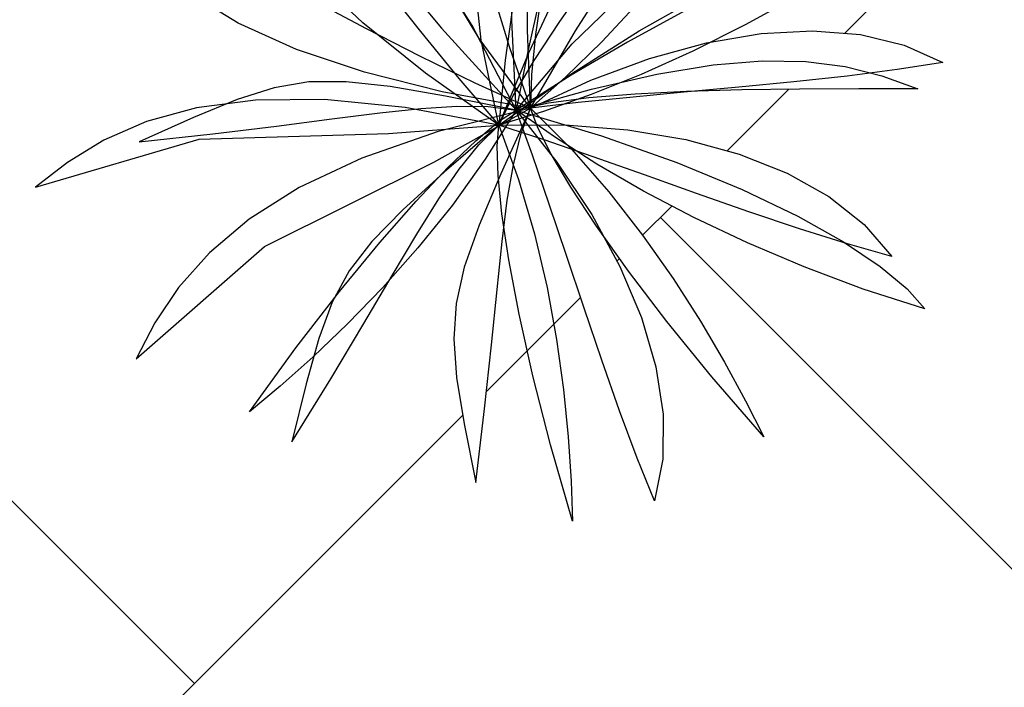
# Model space of a CAD drawing. Units: inches. Extents: x 3590 to 5167, y 65 to 1917.
# Tile 65 of 100: x 4937 to 4968, y 1681 to 1702. Entities that reach past the tile are written whole.
import ezdxf

# ---------------------------------------------------------------- set-up
doc = ezdxf.new("R2010")
doc.units = ezdxf.units.IN
doc.layers.add('A-FLOR-PATT', color=8, linetype='Continuous', lineweight=13)
doc.layers.add('L-PLNT', color=94, linetype='Continuous', lineweight=18)
doc.layers.add('DIENHOA', color=3, linetype='Continuous')

# ---------------------------------------------------------------- blocks, each defined once
blk = doc.blocks.new('Cay03_mb')
at = {"layer": 'DIENHOA'}
for p, q in [((-240.2, 277.8), (-88.4, 94.9)), ((0.2, 104.9), (1.6, 205.7)), ((-49.6, 98.5), (-104.2, 184.4)), ((37.3, 142.1), (20.5, 67.6)), ((75.9, 75.2), (147, 144.1)), ((217.4, 116.6), (145.5, 77.3)), ((5.4, -7.8), (0.2, 104.9)), ((-88.4, 94.9), (5.4, -7.8)), ((5.4, -7.8), (-49.6, 98.5)), ((5.4, -7.8), (75.9, 75.2)), ((145.5, 77.3), (74.7, 36.1)), ((20.5, 67.6), (5.4, -7.8)), ((253, 48.9), (314.6, 54.1)), ((314.6, 54.1), (369.2, 53.3)), ((369.2, 53.3), (418.6, 46.8)), ((100.3, 18.4), (182.2, 37.2)), ((182.2, 37.2), (253, 48.9)), ((418.6, 46.8), (464.9, 35.2)), ((-254.7, 27.4), (-298.6, 20.1)), ((-208, 27.8), (-254.7, 27.4)), ((-152.7, 21.7), (-208, 27.8)), ((74.7, 36.1), (5.4, -7.8)), ((464.9, 35.2), (510, 19)), ((-298.6, 20.1), (-345, 5.4)), ((-83.4, 9.7), (-152.7, 21.7)), ((5.4, -7.8), (100.3, 18.4)), ((219.6, 15.4), (155, 12.2)), ((289, 17.4), (219.6, 15.4)), ((361.6, 18.5), (289, 17.4)), ((435.8, 18.9), (361.6, 18.5)), ((510, 19), (435.8, 18.9)), ((-345, 5.4), (-399.6, -17.1)), ((5.4, -7.8), (-83.4, 9.7)), ((46.3, 0.9), (5.4, -7.8)), ((96.7, 7.5), (46.3, 0.9)), ((155, 12.2), (96.7, 7.5)), ((-225.8, -18.9), (-165.8, -11.3)), ((-165.8, -11.3), (-114, -5.7)), ((-114, -5.7), (-69, -2.9)), ((-69, -2.9), (-29.6, -3.4)), ((5.4, -7.8), (-33.2, -69.5)), ((-29.6, -3.4), (5.4, -7.8)), ((-16.5, -22.4), (5.4, -7.8)), ((5.4, -7.8), (56.8, -73.3)), ((25.9, -64.4), (5.4, -7.8)), ((5.4, -7.8), (112.8, -40.3)), ((53.5, -41.6), (5.4, -7.8)), ((-399.6, -17.1), (-468, -47.9)), ((-295.3, -27.9), (-225.8, -18.9)), ((-45.1, -46.3), (-16.5, -22.4)), ((-375.6, -37.8), (-295.3, -27.9)), ((-468, -47.9), (-375.6, -37.8)), ((-79.8, -79.6), (-45.1, -46.3)), ((107, -75.7), (53.5, -41.6)), ((112.8, -40.3), (207.5, -73.8)), ((-33.2, -69.5), (-74.6, -127.3)), ((47, -125.9), (25.9, -64.4)), ((56.8, -73.3), (100.4, -139.1)), ((207.5, -73.8), (289.5, -107.6)), ((-120.2, -122.1), (-79.8, -79.6)), ((165.5, -109.6), (107, -75.7)), ((228.7, -142.8), (165.5, -109.6)), ((289.5, -107.6), (359.3, -141.1)), ((-165.9, -174.1), (-120.2, -122.1)), ((-74.6, -127.3), (-117.8, -181.1)), ((68.7, -190.6), (47, -125.9)), ((100.4, -139.1), (135.9, -204.3)), ((296, -174.7), (228.7, -142.8)), ((359.3, -141.1), (416.9, -173.5)), ((-216.3, -235.6), (-165.9, -174.1)), ((-117.8, -181.1), (-162.1, -230.9)), ((367.1, -204.8), (296, -174.7)), ((416.9, -173.5), (462.6, -204.2)), ((90.8, -256.6), (68.7, -190.6)), ((135.9, -204.3), (162.8, -268.3)), ((441.6, -232.7), (367.1, -204.8)), ((462.6, -204.2), (496.5, -232.5)), ((-162.1, -230.9), (-206.3, -276.5)), ((518.9, -257.7), (441.6, -232.7)), ((496.5, -232.5), (518.9, -257.7)), ((-271, -306.6), (-216.3, -235.6)), ((113.1, -322.2), (90.8, -256.6)), ((162.8, -268.3), (181, -330.4)), ((-206.3, -276.5), (-249.6, -317.8)), ((-329.5, -387.1), (-271, -306.6)), ((-249.6, -317.8), (-291, -354.7)), ((135.4, -385.6), (113.1, -322.2)), ((181, -330.4), (190, -390)), ((-291, -354.7), (-329.5, -387.1)), ((157.6, -445), (135.4, -385.6)), ((190, -390), (189.6, -446.3)), ((179.5, -498.7), (157.6, -445)), ((189.6, -446.3), (179.5, -498.7))]:
    blk.add_line(p, q, dxfattribs=at)
for points in [[(23.7, -5.4), (-41, 82.2), (-91.8, 167.1), (-129.7, 249.5), (-155.6, 329.6), (-170.2, 407.8), (-174.7, 484.2), (-169.8, 559.3), (-156.5, 633.1)], [(-156.5, 633.1), (-132.5, 551.3), (-110.5, 470), (-89.8, 389.2), (-69.6, 309), (-49, 229.4), (-27.1, 150.4), (-3.2, 72.1), (23.7, -5.4)], [(-16.4, -26.7), (-38.3, 80), (-48.9, 178.3), (-48.7, 269), (-38.5, 352.6), (-19.1, 429.7), (9, 501), (44.9, 567.1), (87.9, 628.5)], [(87.9, 628.5), (75.5, 544.2), (61.3, 461.2), (46.1, 379.1), (30.8, 297.8), (16.1, 216.9), (2.9, 136), (-8.3, 54.9), (-16.4, -26.7)], [(23.7, -5.4), (19.8, 93), (20.3, 177), (25, 248.5), (34, 309.8), (47.3, 362.7), (64.9, 409.3), (86.8, 451.7), (112.9, 491.9)], [(112.9, 491.9), (96, 419.7), (79.5, 347.4), (63.9, 276.5), (50, 208.4), (38.4, 144.8), (29.7, 86.9), (24.6, 36.3), (23.7, -5.4)], [(-395.6, 473.7), (-347.5, 405.6), (-300.6, 339.5), (-254.3, 275.1), (-208.3, 212.3), (-161.9, 150.9), (-114.8, 90.7), (-66.5, 31.6), (-16.4, -26.7)], [(-16.4, -26.7), (-108.3, 38.6), (-186.9, 101.7), (-252.4, 163.5), (-305.1, 224.4), (-345.4, 285.2), (-373.7, 346.6), (-390.4, 409.2), (-395.6, 473.7)], [(384.3, 437.5), (342.2, 367.8), (298.1, 301.7), (252.6, 239.4), (206.1, 181.1), (159.4, 127.2), (113, 78), (67.6, 33.6), (23.7, -5.4)], [(23.7, -5.4), (79.9, 91.7), (134.1, 176.2), (185.8, 248.4), (234.3, 308.7), (279, 357.3), (319.3, 394.8), (354.6, 421.4), (384.3, 437.5)], [(273.2, 387.3), (227.6, 328.8), (182.3, 270.1), (138.4, 212.3), (97.2, 156.4), (60, 103.4), (27.8, 54.6), (1.9, 10.8), (-16.4, -26.7)], [(-16.4, -26.7), (21.4, 64.2), (57, 140.3), (91.4, 203.3), (125.2, 255.1), (159.5, 297.5), (195, 332.5), (232.7, 361.8), (273.2, 387.3)], [(-530.5, 289.7), (-458.3, 248.1), (-387.9, 207.8), (-318.9, 168.7), (-250.8, 131.1), (-182.9, 94.8), (-114.9, 59.9), (-46.2, 26.5), (23.7, -5.4)], [(23.7, -5.4), (-87.2, 15.2), (-185, 39.6), (-270.3, 68.2), (-343.7, 101.4), (-405.9, 139.7), (-457.3, 183.5), (-498.7, 233.4), (-530.5, 289.7)], [(496.7, 224), (429.4, 178.4), (361.6, 136.9), (294.1, 99.5), (227.5, 66.1), (162.4, 36.7), (99.7, 11.5), (39.8, -9.7), (-16.4, -26.7)], [(-16.4, -26.7), (75.4, 37.9), (160.1, 91.8), (237.3, 135.7), (306.6, 170), (367.6, 195.4), (419.9, 212.5), (463.1, 221.9), (496.7, 224)], [(23.7, -5.4), (99.3, 29.7), (173.2, 57.1), (244.8, 76.7), (313.3, 88.3), (377.9, 91.8), (437.9, 87), (492.7, 73.8), (541.4, 52)], [(541.4, 52), (484.1, 42.9), (421.2, 34.8), (354.4, 27.6), (285.4, 20.9), (216.1, 14.5), (148.2, 8.1), (83.5, 1.6), (23.7, -5.4)], [(-16.4, -26.7), (-134, -4.7), (-235.3, 5.3), (-322, 4.7), (-395.9, -5), (-458.7, -22.3), (-512.3, -45.7), (-558.2, -73.6), (-598.4, -104.7)], [(-471.9, -320.3), (-310.5, -179.3), (-97.7, -73.3), (23.7, -5.4)], [(23.7, -5.4), (-92.3, -34.8), (-188.4, -68.2), (-266.9, -105.1), (-329.9, -144.9), (-379.7, -187), (-418.5, -230.7), (-448.5, -275.3), (-471.9, -320.3)], [(23.7, -5.4), (-13.6, -87.9), (-41.1, -152.6), (-59.6, -205), (-69.9, -250.7), (-72.8, -295), (-69.2, -343.6), (-59.7, -401.9), (-45.3, -475.5)], [(-45.3, -475.5), (-34.1, -383.2), (-25.4, -302.8), (-18.3, -233.1), (-12, -172.9), (-5.6, -121.2), (2, -76.8), (11.4, -38.5), (23.7, -5.4)], [(316.5, -418.1), (251.4, -342.8), (194.8, -273.3), (146.5, -210.2), (106.3, -153.8), (74.1, -104.7), (49.7, -63.4), (32.9, -30.1), (23.7, -5.4)], [(23.7, -5.4), (74.9, -57.1), (121.8, -110.6), (164.3, -165), (202.7, -219.4), (237, -272.9), (267.3, -324.5), (293.7, -373.2), (316.5, -418.1)], [(-598.4, -104.7), (-392.7, -44.4), (-155, -37.4), (-16.4, -26.7)], [(-276.2, -424.4), (-227.3, -345.4), (-185.7, -276.1), (-150, -215.7), (-119.1, -163.8), (-91.5, -119.5), (-66, -82.3), (-41.4, -51.6), (-16.4, -26.7)], [(-16.4, -26.7), (-84.9, -86), (-137, -133.1), (-175.8, -173), (-204.3, -210), (-225.5, -249.1), (-242.5, -294.7), (-258.4, -351.6), (-276.2, -424.4)], [(76.2, -524.2), (48.8, -428.5), (26.6, -341.7), (9.2, -264.1), (-3.6, -196.1), (-12.3, -138), (-17.1, -90.2), (-18.3, -53), (-16.4, -26.7)], [(-16.4, -26.7), (66.9, -26.6), (145.6, -32.7), (218.8, -44.9), (285.8, -63.1), (345.9, -87.1), (398.4, -116.6), (442.6, -151.6), (477.6, -191.8)], [(477.6, -191.8), (421.8, -176), (361.3, -156.9), (297.6, -135.5), (232.2, -112.6), (166.6, -89.4), (102.3, -66.6), (40.8, -45.4), (-16.4, -26.7)], [(-16.4, -26.7), (8.5, -95.1), (28.5, -163.3), (44.3, -230.6), (56.3, -296.1), (65, -359), (70.9, -418.5), (74.5, -473.9), (76.2, -524.2)]]:
    blk.add_lwpolyline(points, dxfattribs=at)

msp = doc.modelspace()

# ---------------------------------------------------------------- hatches: boundary and pattern name
at = {"layer": 'A-FLOR-PATT', "transparency": 33554687}
h = msp.add_hatch(dxfattribs=at)
h.set_pattern_fill('AR-HBONE', color=256, scale=0.2)
h.set_pattern_definition([(45, (-588.972, 0), (0, 28.73682), [60.96, -20.32]), (135, (-574.604, 14.368), (3e-15, 28.73682), [60.96, -20.32])])
h.paths.add_polyline_path([(5071.274, 1796.999), (4933.274, 1796.999), (4933.274, 1753.999), (4962.774, 1753.999, -0.414214), (4928.774, 1719.999), (4933.274, 1718.999), (4933.274, 1334.999), (5071.274, 1334.999)])
h.paths.add_polyline_path([(4951.78, 1521.077), (4951.715, 1521.04), (4951.563, 1520.895)], flags=16)
h.paths.add_polyline_path([(4952.267, 1521.376), (4952.198, 1521.371), (4952.198, 1521.356)], flags=0)
h.paths.add_polyline_path([(4967.051, 1529.728), (4965.231, 1528.694), (4963.411, 1527.714), (4961.756, 1526.851), (4963.589, 1527.449), (4964.036, 1527.478), (4962.975, 1527.249), (4961.76, 1526.852), (4959.792, 1525.834), (4958.005, 1524.895), (4956.24, 1523.93), (4954.504, 1522.919), (4954.129, 1522.682), (4953.361, 1521.997), (4953.366, 1521.998), (4953.605, 1522.064), (4955.106, 1522.761), (4956.921, 1523.434), (4958.678, 1523.915), (4960.358, 1524.2), (4961.945, 1524.286), (4964.171, 1524.108), (4965.958, 1523.309), (4963.863, 1522.976), (4965.187, 1522.499), (4963.366, 1522.497), (4961.545, 1522.487), (4959.764, 1522.461), (4958.304, 1522.419), (4957.974, 1522.388), (4956.307, 1522.232), (4954.718, 1522.071), (4953.251, 1521.899), (4953.525, 1521.623), (4954.331, 1521.379), (4956.243, 1521.23), (4958.039, 1520.93), (4959.684, 1520.483), (4961.16, 1519.896), (4963.107, 1518.8), (4964.393, 1517.325), (4962.973, 1517.726), (4964.558, 1516.661), (4965.407, 1515.708), (4963.507, 1516.322), (4961.68, 1517.005), (4959.935, 1517.745), (4958.282, 1518.528), (4956.732, 1519.343), (4955.295, 1520.175), (4954.672, 1520.572), (4954.513, 1520.627), (4955.658, 1519.318), (4956.703, 1517.982), (4957.644, 1516.647), (4958.485, 1515.334), (4959.55, 1513.524), (4960.438, 1511.769), (4958.841, 1513.62), (4957.452, 1515.325), (4955.819, 1517.459), (4956.665, 1515.448), (4957.111, 1513.923), (4957.447, 1511.714), (4957.076, 1509.793), (4956.538, 1511.11), (4955.992, 1512.569), (4955.444, 1514.125), (4954.898, 1515.735), (4954.357, 1517.356), (4953.824, 1518.943), (4953.305, 1520.452), (4953.065, 1521.116), (4952.971, 1521.146), (4952.949, 1521.086), (4952.73, 1520.199), (4953.37, 1518.024), (4953.757, 1516.373), (4954.051, 1514.765), (4954.264, 1513.221), (4954.471, 1511.131), (4954.497, 1510.402), (4954.409, 1511.76), (4954.264, 1513.221), (4954.051, 1514.765), (4953.757, 1516.373), (4953.37, 1518.024), (4952.877, 1519.698), (4952.716, 1520.141), (4952.533, 1519.059), (4952.374, 1517.789), (4952.219, 1516.312), (4952.046, 1514.6), (4951.833, 1512.626), (4951.557, 1510.363), (4951.203, 1512.168), (4950.852, 1514.339), (4950.985, 1516.376), (4951.66, 1518.286), (4952.593, 1520.481), (4952.357, 1521.13), (4951.855, 1520.328), (4950.839, 1518.908), (4949.777, 1517.587), (4948.916, 1516.617), (4948.111, 1515.256), (4947.089, 1513.554), (4945.889, 1511.615), (4946.326, 1513.402), (4946.562, 1514.249), (4945.528, 1513.327), (4944.581, 1512.531), (4946.018, 1514.508), (4947.204, 1516.048), (4947.893, 1517.313), (4949.307, 1518.764), (4950.414, 1519.767), (4950.451, 1519.806), (4952.267, 1521.376), (4951.645, 1521.493), (4950.404, 1521.18), (4948.044, 1520.359), (4946.119, 1519.452), (4944.572, 1518.475), (4943.35, 1517.443), (4941.997, 1515.92), (4941.661, 1515.275), (4942.813, 1516.99), (4944.572, 1518.475), (4946.119, 1519.452), (4948.044, 1520.359), (4950.404, 1521.18), (4951.645, 1521.493), (4949.647, 1521.868), (4948.6, 1521.756), (4947.126, 1521.57), (4945.42, 1521.348), (4943.45, 1521.105), (4941.183, 1520.856), (4942.86, 1521.613), (4943.873, 1522.03), (4942.952, 1521.909), (4941.41, 1521.485), (4939.543, 1520.67), (4938.968, 1520.226), (4940.733, 1521.299), (4942.952, 1521.909), (4943.702, 1522.008), (4945.894, 1522.7), (4947.565, 1522.714), (4948.921, 1522.566), (4951.131, 1522.183), (4950.971, 1522.297), (4948.129, 1523.006), (4946.035, 1523.707), (4944.232, 1524.521), (4942.707, 1525.461), (4941.444, 1526.537), (4940.43, 1527.761), (4939.649, 1529.143), (4941.421, 1528.122), (4943.147, 1527.132), (4944.841, 1526.175), (4946.514, 1525.25), (4948.179, 1524.359), (4948.365, 1524.263), (4946.475, 1526.045), (4945.181, 1527.54), (4944.19, 1529.033), (4943.496, 1530.54), (4943.278, 1531.36), (4942.498, 1531.919), (4943.114, 1531.762), (4942.959, 1533.659), (4944.14, 1531.989), (4944.612, 1531.323), (4946.202, 1530.463), (4947.486, 1529.509), (4948.79, 1528.226), (4950.368, 1526.237), (4949.485, 1528.155), (4948.851, 1530.123), (4948.491, 1532.041), (4948.381, 1533.918), (4948.501, 1535.76), (4948.827, 1537.573), (4949.418, 1535.565), (4949.957, 1533.569), (4950.464, 1531.586), (4950.961, 1529.617), (4951.391, 1527.954), (4951.724, 1530.687), (4952.201, 1532.58), (4952.889, 1534.33), (4953.77, 1535.951), (4954.827, 1537.46), (4954.521, 1535.39), (4954.273, 1533.937), (4955.58, 1535.663), (4956.748, 1536.739), (4956.159, 1534.78), (4955.589, 1532.873), (4955.043, 1531.006), (4954.525, 1529.166), (4954.038, 1527.341), (4953.638, 1525.733), (4953.611, 1525.586), (4953.398, 1524.166), (4953.382, 1524.009), (4954.07, 1525.476), (4954.912, 1527.022), (4956.136, 1528.894), (4957.847, 1530.577), (4959.376, 1531.54), (4958.256, 1530.104), (4957.143, 1528.663), (4956.066, 1527.243), (4955.056, 1525.871), (4954.141, 1524.571), (4953.352, 1523.372), (4953.311, 1523.303), (4953.273, 1522.925), (4953.261, 1522.382), (4954.103, 1523.373), (4954.63, 1524.284), (4955.961, 1526.358), (4957.23, 1528.13), (4958.421, 1529.609), (4960.037, 1531.368), (4961.374, 1532.375), (4962.101, 1532.77), (4961.07, 1531.061), (4959.987, 1529.438), (4958.869, 1527.908), (4958.15, 1527.007), (4959.803, 1528.003), (4961.589, 1528.793), (4963.391, 1529.328), (4965.211, 1529.632)], flags=16)
h.paths.add_polyline_path([(4962.944, 1523.182), (4961.107, 1523.422), (4960.392, 1523.362), (4962.35, 1523.331)], flags=0)
h.paths.add_polyline_path([(5049.541, 1584.551), (5049.476, 1584.515), (5049.325, 1584.37)], flags=16)
h.paths.add_polyline_path([(5050.028, 1584.851), (5049.959, 1584.845), (5049.959, 1584.83)], flags=0)
h.paths.add_polyline_path([(5042.333, 1581.949), (5043.88, 1582.926), (5045.806, 1583.833), (5048.165, 1584.654), (5049.406, 1584.967), (5047.408, 1585.342), (5046.361, 1585.231), (5044.888, 1585.044), (5043.181, 1584.822), (5041.211, 1584.579), (5038.944, 1584.33), (5040.622, 1585.087), (5041.634, 1585.504), (5040.713, 1585.383), (5039.171, 1584.959), (5037.304, 1584.144), (5036.729, 1583.7), (5038.494, 1584.773), (5040.713, 1585.383), (5041.463, 1585.482), (5043.655, 1586.174), (5045.326, 1586.188), (5046.682, 1586.04), (5048.893, 1585.657), (5048.732, 1585.771), (5045.891, 1586.48), (5043.796, 1587.181), (5041.994, 1587.996), (5040.468, 1588.935), (5039.205, 1590.011), (5038.191, 1591.235), (5037.41, 1592.617), (5039.182, 1591.596), (5040.909, 1590.607), (5042.602, 1589.649), (5044.275, 1588.724), (5045.94, 1587.833), (5046.126, 1587.738), (5044.237, 1589.519), (5042.942, 1591.015), (5041.952, 1592.508), (5041.257, 1594.014), (5041.039, 1594.834), (5040.26, 1595.393), (5040.875, 1595.237), (5040.721, 1597.133), (5041.901, 1595.463), (5042.373, 1594.798), (5043.963, 1593.938), (5045.247, 1592.983), (5046.552, 1591.701), (5048.129, 1589.712), (5047.247, 1591.63), (5046.613, 1593.597), (5046.252, 1595.515), (5046.142, 1597.392), (5046.262, 1599.234), (5046.588, 1601.047), (5047.179, 1599.039), (5047.718, 1597.043), (5048.225, 1595.06), (5048.722, 1593.091), (5049.152, 1591.429), (5049.485, 1594.161), (5049.962, 1596.054), (5050.65, 1597.804), (5051.532, 1599.425), (5052.589, 1600.934), (5052.283, 1598.864), (5052.034, 1597.411), (5053.341, 1599.137), (5054.509, 1600.213), (5053.92, 1598.254), (5053.35, 1596.348), (5052.805, 1594.48), (5052.286, 1592.64), (5051.799, 1590.815), (5051.4, 1589.207), (5051.373, 1589.06), (5051.159, 1587.64), (5051.143, 1587.483), (5051.831, 1588.95), (5052.673, 1590.496), (5053.898, 1592.368), (5055.608, 1594.051), (5057.137, 1595.014), (5056.017, 1593.578), (5054.904, 1592.137), (5053.828, 1590.717), (5052.817, 1589.345), (5051.902, 1588.046), (5051.113, 1586.846), (5051.072, 1586.777), (5051.034, 1586.399), (5051.022, 1585.856), (5051.864, 1586.847), (5052.391, 1587.758), (5053.723, 1589.832), (5054.991, 1591.604), (5056.182, 1593.083), (5057.798, 1594.842), (5059.135, 1595.849), (5059.863, 1596.244), (5058.831, 1594.535), (5057.749, 1592.912), (5056.63, 1591.382), (5055.912, 1590.482), (5057.564, 1591.477), (5059.35, 1592.267), (5061.152, 1592.802), (5062.972, 1593.106), (5064.812, 1593.203), (5062.992, 1592.169), (5061.172, 1591.188), (5059.518, 1590.325), (5061.35, 1590.924), (5061.797, 1590.952), (5060.737, 1590.723), (5059.521, 1590.326), (5057.553, 1589.308), (5055.766, 1588.369), (5054.002, 1587.404), (5052.265, 1586.393), (5051.891, 1586.156), (5051.122, 1585.471), (5051.127, 1585.472), (5051.366, 1585.538), (5052.867, 1586.235), (5054.682, 1586.908), (5056.439, 1587.389), (5058.12, 1587.675), (5059.706, 1587.76), (5061.933, 1587.583), (5063.719, 1586.783), (5061.624, 1586.45), (5062.949, 1585.973), (5061.127, 1585.971), (5059.307, 1585.961), (5057.525, 1585.935), (5056.065, 1585.893), (5055.735, 1585.862), (5054.068, 1585.707), (5052.479, 1585.546), (5051.012, 1585.373), (5051.286, 1585.097), (5052.092, 1584.853), (5054.004, 1584.704), (5055.8, 1584.404), (5057.446, 1583.958), (5058.921, 1583.37), (5060.868, 1582.274), (5062.154, 1580.799), (5060.734, 1581.2), (5062.32, 1580.135), (5063.168, 1579.182), (5061.269, 1579.796), (5059.441, 1580.479), (5057.696, 1581.219), (5056.043, 1582.003), (5054.493, 1582.817), (5053.057, 1583.649), (5052.433, 1584.047), (5052.274, 1584.101), (5053.42, 1582.793), (5054.464, 1581.457), (5055.405, 1580.121), (5056.247, 1578.809), (5057.311, 1576.998), (5058.199, 1575.244), (5056.602, 1577.094), (5055.213, 1578.799), (5053.58, 1580.933), (5054.427, 1578.922), (5054.872, 1577.397), (5055.208, 1575.189), (5054.838, 1573.267), (5054.299, 1574.584), (5053.754, 1576.043), (5053.206, 1577.599), (5052.659, 1579.209), (5052.118, 1580.83), (5051.585, 1582.417), (5051.066, 1583.927), (5050.826, 1584.59), (5050.733, 1584.62), (5050.711, 1584.561), (5050.491, 1583.673), (5051.131, 1581.498), (5051.518, 1579.847), (5051.813, 1578.24), (5052.026, 1576.695), (5052.233, 1574.605), (5052.258, 1573.876), (5052.17, 1575.234), (5052.026, 1576.695), (5051.813, 1578.24), (5051.518, 1579.847), (5051.131, 1581.498), (5050.638, 1583.172), (5050.477, 1583.615), (5050.294, 1582.533), (5050.136, 1581.263), (5049.981, 1579.786), (5049.807, 1578.074), (5049.594, 1576.1), (5049.318, 1573.837), (5048.965, 1575.642), (5048.613, 1577.813), (5048.747, 1579.85), (5049.421, 1581.76), (5050.354, 1583.955), (5050.118, 1584.604), (5049.616, 1583.802), (5048.6, 1582.382), (5047.538, 1581.061), (5046.677, 1580.091), (5045.872, 1578.73), (5044.85, 1577.028), (5043.651, 1575.089), (5044.087, 1576.877), (5044.324, 1577.723), (5043.289, 1576.801), (5042.342, 1576.005), (5043.779, 1577.982), (5044.966, 1579.522), (5045.655, 1580.787), (5047.068, 1582.239), (5048.175, 1583.241), (5048.213, 1583.28), (5050.028, 1584.851), (5049.406, 1584.967), (5048.165, 1584.654), (5045.806, 1583.833), (5043.88, 1582.926), (5042.333, 1581.949), (5041.111, 1580.917), (5039.758, 1579.394), (5039.423, 1578.749), (5040.575, 1580.464)], flags=16)
h.paths.add_polyline_path([(4954.799, 1533.12), (4954.262, 1532.079), (4953.831, 1530.935), (4953.505, 1529.636), (4953.283, 1528.133), (4953.167, 1526.376), (4953.156, 1524.315), (4953.277, 1521.236), (4952.802, 1521.842), (4951.557, 1521.998), (4950.976, 1521.961), (4952.661, 1521.941), (4952.802, 1521.842), (4953.152, 1523.593), (4953.167, 1526.376), (4953.283, 1528.133), (4953.609, 1530.346), (4954.456, 1532.592)], flags=0)
h.paths.add_polyline_path([(5050.563, 1585.316), (5049.318, 1585.472), (5048.737, 1585.435), (5050.422, 1585.415), (5050.563, 1585.316), (5050.914, 1587.067), (5050.928, 1589.851), (5051.045, 1591.607), (5051.371, 1593.82), (5052.217, 1596.066), (5052.56, 1596.594), (5052.024, 1595.554), (5051.592, 1594.409), (5051.266, 1593.11), (5051.045, 1591.607), (5050.928, 1589.851), (5050.918, 1587.789), (5051.038, 1584.71)], flags=0)
h.paths.add_polyline_path([(5058.153, 1586.836), (5060.111, 1586.805), (5060.705, 1586.656), (5058.868, 1586.896)], flags=0)
h.paths.add_polyline_path([(5049.541, 1430.936), (5049.476, 1430.9), (5049.325, 1430.755)], flags=16)
h.paths.add_polyline_path([(5050.028, 1431.236), (5049.959, 1431.231), (5049.959, 1431.215)], flags=0)
h.paths.add_polyline_path([(5046.588, 1447.432), (5047.179, 1445.425), (5047.718, 1443.429), (5048.225, 1441.446), (5048.722, 1439.476), (5049.152, 1437.814), (5049.485, 1440.546), (5049.962, 1442.439), (5050.65, 1444.189), (5051.532, 1445.811), (5052.589, 1447.319), (5052.283, 1445.249), (5052.034, 1443.796), (5053.341, 1445.522), (5054.509, 1446.598), (5053.92, 1444.64), (5053.35, 1442.733), (5052.805, 1440.865), (5052.286, 1439.025), (5051.799, 1437.201), (5051.4, 1435.592), (5051.373, 1435.445), (5051.159, 1434.025), (5051.143, 1433.868), (5051.831, 1435.335), (5052.673, 1436.881), (5053.898, 1438.753), (5055.608, 1440.436), (5057.137, 1441.4), (5056.017, 1439.963), (5054.904, 1438.522), (5053.828, 1437.102), (5052.817, 1435.73), (5051.902, 1434.431), (5051.113, 1433.231), (5051.072, 1433.162), (5051.034, 1432.784), (5051.022, 1432.242), (5051.864, 1433.232), (5052.391, 1434.143), (5053.723, 1436.217), (5054.991, 1437.989), (5056.182, 1439.468), (5057.798, 1441.227), (5059.135, 1442.235), (5059.863, 1442.629), (5058.831, 1440.921), (5057.749, 1439.298), (5056.63, 1437.767), (5055.912, 1436.867), (5057.564, 1437.863), (5059.35, 1438.652), (5061.152, 1439.187), (5062.972, 1439.491), (5064.812, 1439.588), (5062.992, 1438.554), (5061.172, 1437.573), (5059.518, 1436.71), (5061.35, 1437.309), (5061.797, 1437.337), (5060.737, 1437.108), (5059.521, 1436.711), (5057.553, 1435.693), (5055.766, 1434.754), (5054.002, 1433.789), (5052.265, 1432.778), (5051.891, 1432.541), (5051.122, 1431.856), (5051.127, 1431.857), (5051.366, 1431.923), (5052.867, 1432.62), (5054.682, 1433.293), (5056.439, 1433.775), (5058.12, 1434.06), (5059.706, 1434.145), (5061.933, 1433.968), (5063.719, 1433.168), (5061.624, 1432.835), (5062.949, 1432.358), (5061.127, 1432.357), (5059.307, 1432.346), (5057.525, 1432.32), (5056.065, 1432.278), (5055.735, 1432.248), (5054.068, 1432.092), (5052.479, 1431.931), (5051.012, 1431.759), (5051.286, 1431.482), (5052.092, 1431.238), (5054.004, 1431.089), (5055.8, 1430.789), (5057.446, 1430.343), (5058.921, 1429.755), (5060.868, 1428.66), (5062.154, 1427.185), (5060.734, 1427.585), (5062.32, 1426.52), (5063.168, 1425.567), (5061.269, 1426.181), (5059.441, 1426.865), (5057.696, 1427.604), (5056.043, 1428.388), (5054.493, 1429.202), (5053.057, 1430.034), (5052.433, 1430.432), (5052.274, 1430.487), (5053.42, 1429.178), (5054.464, 1427.842), (5055.405, 1426.506), (5056.247, 1425.194), (5057.311, 1423.383), (5058.199, 1421.629), (5056.602, 1423.479), (5055.213, 1425.184), (5053.58, 1427.318), (5054.427, 1425.307), (5054.872, 1423.782), (5055.208, 1421.574), (5054.838, 1419.652), (5054.299, 1420.97), (5053.754, 1422.428), (5053.206, 1423.984), (5052.659, 1425.595), (5052.118, 1427.215), (5051.585, 1428.802), (5051.066, 1430.312), (5050.826, 1430.975), (5050.733, 1431.005), (5050.711, 1430.946), (5050.491, 1430.058), (5051.131, 1427.883), (5051.518, 1426.232), (5051.813, 1424.625), (5052.026, 1423.081), (5052.233, 1420.991), (5052.258, 1420.261), (5052.17, 1421.619), (5052.026, 1423.081), (5051.813, 1424.625), (5051.518, 1426.232), (5051.131, 1427.883), (5050.638, 1429.558), (5050.477, 1430.001), (5050.294, 1428.918), (5050.136, 1427.648), (5049.981, 1426.171), (5049.807, 1424.459), (5049.594, 1422.485), (5049.318, 1420.222), (5048.965, 1422.028), (5048.613, 1424.199), (5048.747, 1426.235), (5049.421, 1428.146), (5050.354, 1430.34), (5050.118, 1430.989), (5049.616, 1430.187), (5048.6, 1428.768), (5047.538, 1427.446), (5046.677, 1426.477), (5045.872, 1425.116), (5044.85, 1423.413), (5043.651, 1421.474), (5044.087, 1423.262), (5044.324, 1424.109), (5043.289, 1423.186), (5042.342, 1422.391), (5043.779, 1424.368), (5044.966, 1425.907), (5045.655, 1427.173), (5047.068, 1428.624), (5048.175, 1429.627), (5048.213, 1429.666), (5050.028, 1431.236), (5049.406, 1431.353), (5048.165, 1431.039), (5045.806, 1430.218), (5043.88, 1429.311), (5042.333, 1428.334), (5041.111, 1427.302), (5039.758, 1425.779), (5039.423, 1425.134), (5040.575, 1426.849), (5042.333, 1428.334), (5043.88, 1429.311), (5045.806, 1430.218), (5048.165, 1431.039), (5049.406, 1431.353), (5047.408, 1431.727), (5046.361, 1431.616), (5044.888, 1431.429), (5043.181, 1431.207), (5041.211, 1430.964), (5038.944, 1430.715), (5040.622, 1431.472), (5041.634, 1431.89), (5040.713, 1431.769), (5039.171, 1431.345), (5037.304, 1430.53), (5036.729, 1430.085), (5038.494, 1431.158), (5040.713, 1431.769), (5041.463, 1431.867), (5043.655, 1432.559), (5045.326, 1432.573), (5046.682, 1432.425), (5048.893, 1432.042), (5048.732, 1432.156), (5045.891, 1432.865), (5043.796, 1433.566), (5041.994, 1434.381), (5040.468, 1435.321), (5039.205, 1436.396), (5038.191, 1437.62), (5037.41, 1439.002), (5039.182, 1437.982), (5040.909, 1436.992), (5042.602, 1436.034), (5044.275, 1435.109), (5045.94, 1434.218), (5046.126, 1434.123), (5044.237, 1435.904), (5042.942, 1437.4), (5041.952, 1438.893), (5041.257, 1440.399), (5041.039, 1441.219), (5040.26, 1441.778), (5040.875, 1441.622), (5040.721, 1443.518), (5041.901, 1441.848), (5042.373, 1441.183), (5043.963, 1440.323), (5045.247, 1439.369), (5046.552, 1438.086), (5048.129, 1436.097), (5047.247, 1438.015), (5046.613, 1439.982), (5046.252, 1441.901), (5046.142, 1443.778), (5046.262, 1445.619)], flags=16)
h.paths.add_polyline_path([(5052.382, 1444.255), (5051.623, 1442.78), (5052.024, 1441.939), (5052.56, 1442.98)], flags=0)
h.paths.add_polyline_path([(5050.563, 1431.701), (5049.318, 1431.857), (5048.737, 1431.821), (5050.422, 1431.8)], flags=0)
h.paths.add_polyline_path([(5058.153, 1433.221), (5060.111, 1433.19), (5060.705, 1433.041), (5058.868, 1433.281)], flags=0)
h.paths.add_polyline_path([(5049.541, 1352.285), (5049.476, 1352.249), (5049.325, 1352.104)], flags=16)
h.paths.add_polyline_path([(5050.028, 1352.585), (5049.959, 1352.58), (5049.959, 1352.564)], flags=0)
h.paths.add_polyline_path([(5046.588, 1368.781), (5047.179, 1366.774), (5047.718, 1364.778), (5048.225, 1362.795), (5048.722, 1360.825), (5049.152, 1359.163), (5049.485, 1361.896), (5049.962, 1363.789), (5050.65, 1365.538), (5051.532, 1367.16), (5052.589, 1368.669), (5052.283, 1366.598), (5052.034, 1365.145), (5053.341, 1366.871), (5054.509, 1367.947), (5053.92, 1365.989), (5053.35, 1364.082), (5052.805, 1362.214), (5052.286, 1360.374), (5051.799, 1358.55), (5051.4, 1356.942), (5051.373, 1356.794), (5051.159, 1355.374), (5051.143, 1355.218), (5051.831, 1356.684), (5052.673, 1358.23), (5053.898, 1360.102), (5055.608, 1361.786), (5057.137, 1362.749), (5056.017, 1361.313), (5054.904, 1359.872), (5053.828, 1358.452), (5052.817, 1357.079), (5051.902, 1355.78), (5051.113, 1354.581), (5051.072, 1354.512), (5051.034, 1354.133), (5051.022, 1353.591), (5051.864, 1354.581), (5052.391, 1355.492), (5053.723, 1357.566), (5054.991, 1359.338), (5056.182, 1360.817), (5057.798, 1362.577), (5059.135, 1363.584), (5059.863, 1363.979), (5058.831, 1362.27), (5057.749, 1360.647), (5056.63, 1359.117), (5055.912, 1358.216), (5057.564, 1359.212), (5059.35, 1360.001), (5061.152, 1360.536), (5062.972, 1360.841), (5064.812, 1360.937), (5062.992, 1359.903), (5061.172, 1358.923), (5059.518, 1358.059), (5061.35, 1358.658), (5061.797, 1358.687), (5060.737, 1358.458), (5059.521, 1358.061), (5057.553, 1357.043), (5055.766, 1356.103), (5054.002, 1355.138), (5052.265, 1354.127), (5051.891, 1353.89), (5051.122, 1353.206), (5051.127, 1353.206), (5051.366, 1353.272), (5052.867, 1353.969), (5054.682, 1354.643), (5056.439, 1355.124), (5058.12, 1355.409), (5059.706, 1355.495), (5061.933, 1355.317), (5063.719, 1354.518), (5061.624, 1354.184), (5062.949, 1353.708), (5061.127, 1353.706), (5059.307, 1353.695), (5057.525, 1353.669), (5056.065, 1353.627), (5055.735, 1353.597), (5054.068, 1353.441), (5052.479, 1353.28), (5051.012, 1353.108), (5051.286, 1352.831), (5052.092, 1352.587), (5054.004, 1352.439), (5055.8, 1352.138), (5057.446, 1351.692), (5058.921, 1351.104), (5060.868, 1350.009), (5062.154, 1348.534), (5060.734, 1348.935), (5062.32, 1347.869), (5063.168, 1346.916), (5061.269, 1347.53), (5059.441, 1348.214), (5057.696, 1348.954), (5056.043, 1349.737), (5054.493, 1350.551), (5053.057, 1351.383), (5052.433, 1351.781), (5052.274, 1351.836), (5053.42, 1350.527), (5054.464, 1349.191), (5055.405, 1347.855), (5056.247, 1346.543), (5057.311, 1344.733), (5058.199, 1342.978), (5056.602, 1344.828), (5055.213, 1346.534), (5053.58, 1348.667), (5054.427, 1346.656), (5054.872, 1345.132), (5055.208, 1342.923), (5054.838, 1341.002), (5054.299, 1342.319), (5053.754, 1343.778), (5053.206, 1345.334), (5052.659, 1346.944), (5052.118, 1348.564), (5051.585, 1350.151), (5051.066, 1351.661), (5050.826, 1352.324), (5050.733, 1352.355), (5050.711, 1352.295), (5050.491, 1351.408), (5051.131, 1349.232), (5051.518, 1347.581), (5051.813, 1345.974), (5052.026, 1344.43), (5052.233, 1342.34), (5052.258, 1341.61), (5052.17, 1342.969), (5052.026, 1344.43), (5051.813, 1345.974), (5051.518, 1347.581), (5051.131, 1349.232), (5050.638, 1350.907), (5050.477, 1351.35), (5050.294, 1350.267), (5050.136, 1348.997), (5049.981, 1347.52), (5049.807, 1345.809), (5049.594, 1343.835), (5049.318, 1341.571), (5048.965, 1343.377), (5048.613, 1345.548), (5048.747, 1347.585), (5049.421, 1349.495), (5050.354, 1351.689), (5050.118, 1352.339), (5049.616, 1351.536), (5048.6, 1350.117), (5047.538, 1348.795), (5046.677, 1347.826), (5045.872, 1346.465), (5044.85, 1344.763), (5043.651, 1342.824), (5044.087, 1344.611), (5044.324, 1345.458), (5043.289, 1344.535), (5042.342, 1343.74), (5043.779, 1345.717), (5044.966, 1347.256), (5045.655, 1348.522), (5047.068, 1349.973), (5048.175, 1350.976), (5048.213, 1351.015), (5050.028, 1352.585), (5049.406, 1352.702), (5048.165, 1352.388), (5045.806, 1351.567), (5043.88, 1350.661), (5042.333, 1349.683), (5041.111, 1348.651), (5039.758, 1347.128), (5039.423, 1346.483), (5040.575, 1348.198), (5042.333, 1349.683), (5043.88, 1350.661), (5045.806, 1351.567), (5048.165, 1352.388), (5049.406, 1352.702), (5047.408, 1353.076), (5046.361, 1352.965), (5044.888, 1352.779), (5043.181, 1352.556), (5041.211, 1352.313), (5038.944, 1352.065), (5040.622, 1352.821), (5041.634, 1353.239), (5040.713, 1353.118), (5039.171, 1352.694), (5037.304, 1351.879), (5036.729, 1351.434), (5038.494, 1352.508), (5040.713, 1353.118), (5041.463, 1353.216), (5043.655, 1353.909), (5045.326, 1353.923), (5046.682, 1353.774), (5048.893, 1353.391), (5048.732, 1353.506), (5045.891, 1354.214), (5043.796, 1354.915), (5041.994, 1355.73), (5040.468, 1356.67), (5039.205, 1357.746), (5038.191, 1358.969), (5037.41, 1360.352), (5039.182, 1359.331), (5040.909, 1358.341), (5042.602, 1357.383), (5044.275, 1356.458), (5045.94, 1355.567), (5046.126, 1355.472), (5044.237, 1357.253), (5042.942, 1358.749), (5041.952, 1360.242), (5041.257, 1361.748), (5041.039, 1362.568), (5040.26, 1363.128), (5040.875, 1362.971), (5040.721, 1364.867), (5041.901, 1363.197), (5042.373, 1362.532), (5043.963, 1361.672), (5045.247, 1360.718), (5046.552, 1359.435), (5048.129, 1357.446), (5047.247, 1359.364), (5046.613, 1361.331), (5046.252, 1363.25), (5046.142, 1365.127), (5046.262, 1366.969)], flags=16)
h.paths.add_polyline_path([(5052.382, 1365.604), (5051.623, 1364.129), (5052.024, 1363.288), (5052.56, 1364.329)], flags=0)
h.paths.add_polyline_path([(4951.78, 1698.041), (4951.715, 1698.005), (4951.563, 1697.859)], flags=16)
h.paths.add_polyline_path([(4952.267, 1698.341), (4952.198, 1698.335), (4952.198, 1698.32)], flags=0)
h.paths.add_polyline_path([(4957.076, 1686.757), (4956.538, 1688.074), (4955.992, 1689.533), (4955.444, 1691.089), (4954.898, 1692.699), (4954.357, 1694.32), (4953.824, 1695.907), (4953.305, 1697.417), (4953.065, 1698.08), (4952.971, 1698.11), (4952.949, 1698.051), (4952.73, 1697.163), (4953.37, 1694.988), (4953.757, 1693.337), (4954.051, 1691.729), (4954.264, 1690.185), (4954.471, 1688.095), (4954.497, 1687.366), (4954.409, 1688.724), (4954.264, 1690.185), (4954.051, 1691.729), (4953.757, 1693.337), (4953.37, 1694.988), (4952.877, 1696.662), (4952.716, 1697.105), (4952.533, 1696.023), (4952.374, 1694.753), (4952.219, 1693.276), (4952.046, 1691.564), (4951.833, 1689.59), (4951.557, 1687.327), (4951.203, 1689.132), (4950.852, 1691.303), (4950.985, 1693.34), (4951.66, 1695.25), (4952.593, 1697.445), (4952.357, 1698.094), (4951.855, 1697.292), (4950.839, 1695.872), (4949.777, 1694.551), (4948.916, 1693.581), (4948.111, 1692.22), (4947.089, 1690.518), (4945.889, 1688.579), (4946.326, 1690.366), (4946.562, 1691.213), (4945.528, 1690.291), (4944.581, 1689.495), (4946.018, 1691.472), (4947.204, 1693.012), (4947.893, 1694.277), (4949.307, 1695.729), (4950.414, 1696.731), (4950.451, 1696.77), (4952.267, 1698.341), (4951.645, 1698.457), (4950.404, 1698.144), (4948.044, 1697.323), (4946.119, 1696.416), (4944.572, 1695.439), (4943.35, 1694.407), (4941.997, 1692.884), (4941.661, 1692.239), (4942.813, 1693.954), (4944.572, 1695.439), (4946.119, 1696.416), (4948.044, 1697.323), (4950.404, 1698.144), (4951.645, 1698.457), (4949.647, 1698.832), (4948.6, 1698.72), (4947.126, 1698.534), (4945.42, 1698.312), (4943.45, 1698.069), (4941.183, 1697.82), (4942.86, 1698.577), (4943.873, 1698.994), (4942.952, 1698.873), (4941.41, 1698.449), (4939.543, 1697.634), (4938.968, 1697.19), (4940.733, 1698.263), (4942.952, 1698.873), (4943.702, 1698.972), (4945.894, 1699.664), (4947.565, 1699.678), (4948.921, 1699.53), (4951.131, 1699.147), (4950.971, 1699.261), (4948.129, 1699.97), (4946.035, 1700.671), (4944.232, 1701.486), (4942.707, 1702.425), (4941.444, 1703.501), (4940.43, 1704.725), (4939.649, 1706.107), (4941.421, 1705.086), (4943.147, 1704.097), (4944.841, 1703.139), (4946.514, 1702.214), (4948.179, 1701.323), (4948.365, 1701.227), (4946.475, 1703.009), (4945.181, 1704.505), (4944.19, 1705.997), (4943.496, 1707.504), (4943.278, 1708.324), (4942.498, 1708.883), (4943.114, 1708.727), (4942.959, 1710.623), (4944.14, 1708.953), (4944.612, 1708.287), (4946.202, 1707.428), (4947.486, 1706.473), (4948.79, 1705.191), (4950.368, 1703.202), (4949.485, 1705.12), (4948.851, 1707.087), (4948.491, 1709.005), (4948.381, 1710.882), (4948.501, 1712.724), (4948.827, 1714.537), (4949.418, 1712.529), (4949.957, 1710.533), (4950.464, 1708.55), (4950.961, 1706.581), (4951.391, 1704.919), (4951.724, 1707.651), (4952.201, 1709.544), (4952.889, 1711.294), (4953.77, 1712.915), (4954.827, 1714.424), (4954.521, 1712.354), (4954.273, 1710.901), (4955.58, 1712.627), (4956.748, 1713.703), (4956.159, 1711.744), (4955.589, 1709.837), (4955.043, 1707.97), (4954.525, 1706.13), (4954.038, 1704.305), (4953.638, 1702.697), (4953.611, 1702.55), (4953.398, 1701.13), (4953.382, 1700.973), (4954.07, 1702.44), (4954.912, 1703.986), (4956.136, 1705.858), (4957.847, 1707.541), (4959.376, 1708.504), (4958.256, 1707.068), (4957.143, 1705.627), (4956.066, 1704.207), (4955.056, 1702.835), (4954.141, 1701.536), (4953.352, 1700.336), (4953.311, 1700.267), (4953.273, 1699.889), (4953.261, 1699.346), (4954.103, 1700.337), (4954.63, 1701.248), (4955.961, 1703.322), (4957.23, 1705.094), (4958.421, 1706.573), (4960.037, 1708.332), (4961.374, 1709.339), (4962.101, 1709.734), (4961.07, 1708.025), (4959.987, 1706.402), (4958.869, 1704.872), (4958.15, 1703.972), (4959.803, 1704.967), (4961.589, 1705.757), (4963.391, 1706.292), (4965.211, 1706.596), (4967.051, 1706.692), (4965.231, 1705.659), (4963.411, 1704.678), (4961.756, 1703.815), (4963.589, 1704.413), (4964.036, 1704.442), (4962.975, 1704.213), (4961.76, 1703.816), (4959.792, 1702.798), (4958.005, 1701.859), (4956.24, 1700.894), (4954.504, 1699.883), (4954.129, 1699.646), (4953.361, 1698.961), (4953.366, 1698.962), (4953.605, 1699.028), (4955.106, 1699.725), (4956.921, 1700.398), (4958.678, 1700.879), (4960.358, 1701.164), (4961.945, 1701.25), (4964.171, 1701.073), (4965.958, 1700.273), (4963.863, 1699.94), (4965.187, 1699.463), (4963.366, 1699.461), (4961.545, 1699.451), (4959.764, 1699.425), (4958.304, 1699.383), (4957.974, 1699.352), (4956.307, 1699.197), (4954.718, 1699.036), (4953.251, 1698.863), (4953.525, 1698.587), (4954.331, 1698.343), (4956.243, 1698.194), (4958.039, 1697.894), (4959.684, 1697.447), (4961.16, 1696.86), (4963.107, 1695.764), (4964.393, 1694.289), (4962.973, 1694.69), (4964.558, 1693.625), (4965.407, 1692.672), (4963.507, 1693.286), (4961.68, 1693.969), (4959.935, 1694.709), (4958.282, 1695.492), (4956.732, 1696.307), (4955.295, 1697.139), (4954.672, 1697.536), (4954.513, 1697.591), (4955.658, 1696.282), (4956.703, 1694.946), (4957.644, 1693.611), (4958.485, 1692.298), (4959.55, 1690.488), (4960.438, 1688.733), (4958.841, 1690.584), (4957.452, 1692.289), (4955.819, 1694.423), (4956.665, 1692.412), (4957.111, 1690.887), (4957.447, 1688.678)], flags=16)
h.paths.add_polyline_path([(5050.563, 1353.05), (5049.318, 1353.207), (5048.737, 1353.17), (5050.422, 1353.15)], flags=0)
h.paths.add_polyline_path([(4951.78, 1351.486), (4951.715, 1351.45), (4951.563, 1351.305)], flags=16)
h.paths.add_polyline_path([(4952.267, 1351.786), (4952.198, 1351.78), (4952.198, 1351.765)], flags=0)
h.paths.add_polyline_path([(4954.827, 1367.869), (4954.521, 1365.799), (4954.273, 1364.346), (4955.58, 1366.072), (4956.748, 1367.148), (4956.159, 1365.19), (4955.589, 1363.283), (4955.043, 1361.415), (4954.525, 1359.575), (4954.038, 1357.751), (4953.638, 1356.142), (4953.611, 1355.995), (4953.398, 1354.575), (4953.382, 1354.418), (4954.07, 1355.885), (4954.912, 1357.431), (4956.136, 1359.303), (4957.847, 1360.986), (4959.376, 1361.95), (4958.256, 1360.513), (4957.143, 1359.072), (4956.066, 1357.652), (4955.056, 1356.28), (4954.141, 1354.981), (4953.352, 1353.781), (4953.311, 1353.712), (4953.273, 1353.334), (4953.261, 1352.792), (4954.103, 1353.782), (4954.63, 1354.693), (4955.961, 1356.767), (4957.23, 1358.539), (4958.421, 1360.018), (4960.037, 1361.777), (4961.374, 1362.785), (4962.101, 1363.179), (4961.07, 1361.471), (4959.987, 1359.848), (4958.869, 1358.317), (4958.15, 1357.417), (4959.803, 1358.413), (4961.589, 1359.202), (4963.391, 1359.737), (4965.211, 1360.041), (4967.051, 1360.138), (4965.231, 1359.104), (4963.411, 1358.123), (4961.756, 1357.26), (4963.589, 1357.859), (4964.036, 1357.887), (4962.975, 1357.658), (4961.76, 1357.261), (4959.792, 1356.243), (4958.005, 1355.304), (4956.24, 1354.339), (4954.504, 1353.328), (4954.129, 1353.091), (4953.361, 1352.406), (4953.366, 1352.407), (4953.605, 1352.473), (4955.106, 1353.17), (4956.921, 1353.843), (4958.678, 1354.325), (4960.358, 1354.61), (4961.945, 1354.695), (4964.171, 1354.518), (4965.958, 1353.718), (4963.863, 1353.385), (4965.187, 1352.908), (4963.366, 1352.907), (4961.545, 1352.896), (4959.764, 1352.87), (4958.304, 1352.828), (4957.974, 1352.798), (4956.307, 1352.642), (4954.718, 1352.481), (4953.251, 1352.309), (4953.525, 1352.032), (4954.331, 1351.788), (4956.243, 1351.639), (4958.039, 1351.339), (4959.684, 1350.893), (4961.16, 1350.305), (4963.107, 1349.21), (4964.393, 1347.735), (4962.973, 1348.135), (4964.558, 1347.07), (4965.407, 1346.117), (4963.507, 1346.731), (4961.68, 1347.414), (4959.935, 1348.154), (4958.282, 1348.938), (4956.732, 1349.752), (4955.295, 1350.584), (4954.672, 1350.982), (4954.513, 1351.036), (4955.658, 1349.728), (4956.703, 1348.392), (4957.644, 1347.056), (4958.485, 1345.744), (4959.55, 1343.933), (4960.438, 1342.179), (4958.841, 1344.029), (4957.452, 1345.734), (4955.819, 1347.868), (4956.665, 1345.857), (4957.111, 1344.332), (4957.447, 1342.124), (4957.076, 1340.202), (4956.538, 1341.52), (4955.992, 1342.978), (4955.444, 1344.534), (4954.898, 1346.145), (4954.357, 1347.765), (4953.824, 1349.352), (4953.305, 1350.862), (4953.065, 1351.525), (4952.971, 1351.555), (4952.949, 1351.496), (4952.73, 1350.608), (4953.37, 1348.433), (4953.757, 1346.782), (4954.051, 1345.175), (4954.264, 1343.631), (4954.471, 1341.541), (4954.497, 1340.811), (4954.409, 1342.169), (4954.264, 1343.631), (4954.051, 1345.175), (4953.757, 1346.782), (4953.37, 1348.433), (4952.877, 1350.108), (4952.716, 1350.551), (4952.533, 1349.468), (4952.374, 1348.198), (4952.219, 1346.721), (4952.046, 1345.009), (4951.833, 1343.035), (4951.557, 1340.772), (4951.203, 1342.578), (4950.852, 1344.749), (4950.985, 1346.785), (4951.66, 1348.696), (4952.593, 1350.89), (4952.357, 1351.539), (4951.855, 1350.737), (4950.839, 1349.318), (4949.777, 1347.996), (4948.916, 1347.027), (4948.111, 1345.665), (4947.089, 1343.963), (4945.889, 1342.024), (4946.326, 1343.812), (4946.562, 1344.659), (4945.528, 1343.736), (4944.581, 1342.941), (4946.018, 1344.918), (4947.204, 1346.457), (4947.893, 1347.723), (4949.307, 1349.174), (4950.414, 1350.177), (4950.451, 1350.216), (4952.267, 1351.786), (4951.645, 1351.903), (4950.404, 1351.589), (4948.044, 1350.768), (4946.119, 1349.861), (4944.572, 1348.884), (4943.35, 1347.852), (4941.997, 1346.329), (4941.661, 1345.684), (4942.813, 1347.399), (4944.572, 1348.884), (4946.119, 1349.861), (4948.044, 1350.768), (4950.404, 1351.589), (4951.645, 1351.903), (4949.647, 1352.277), (4948.6, 1352.166), (4947.126, 1351.979), (4945.42, 1351.757), (4943.45, 1351.514), (4941.183, 1351.265), (4942.86, 1352.022), (4943.873, 1352.44), (4942.952, 1352.319), (4941.41, 1351.895), (4939.543, 1351.08), (4938.968, 1350.635), (4940.733, 1351.708), (4942.952, 1352.319), (4943.702, 1352.417), (4945.894, 1353.109), (4947.565, 1353.123), (4948.921, 1352.975), (4951.131, 1352.592), (4950.971, 1352.706), (4948.129, 1353.415), (4946.035, 1354.116), (4944.232, 1354.931), (4942.707, 1355.871), (4941.444, 1356.946), (4940.43, 1358.17), (4939.649, 1359.552), (4941.421, 1358.532), (4943.147, 1357.542), (4944.841, 1356.584), (4946.514, 1355.659), (4948.179, 1354.768), (4948.365, 1354.673), (4946.475, 1356.454), (4945.181, 1357.95), (4944.19, 1359.443), (4943.496, 1360.949), (4943.278, 1361.769), (4942.498, 1362.328), (4943.114, 1362.172), (4942.959, 1364.068), (4944.14, 1362.398), (4944.612, 1361.733), (4946.202, 1360.873), (4947.486, 1359.919), (4948.79, 1358.636), (4950.368, 1356.647), (4949.485, 1358.565), (4948.851, 1360.532), (4948.491, 1362.451), (4948.381, 1364.328), (4948.501, 1366.169), (4948.827, 1367.982), (4949.418, 1365.975), (4949.957, 1363.979), (4950.464, 1361.995), (4950.961, 1360.026), (4951.391, 1358.364), (4951.724, 1361.096), (4952.201, 1362.989), (4952.889, 1364.739), (4953.77, 1366.361)], flags=16)
h.paths.add_polyline_path([(4954.799, 1363.53), (4954.262, 1362.489), (4953.831, 1361.344), (4953.505, 1360.045), (4953.283, 1358.543), (4953.167, 1356.786), (4953.156, 1354.724), (4953.277, 1351.646), (4952.802, 1352.251), (4951.557, 1352.407), (4950.976, 1352.371), (4952.661, 1352.35), (4952.802, 1352.251), (4953.152, 1354.002), (4953.167, 1356.786), (4953.283, 1358.543), (4953.609, 1360.755), (4954.456, 1363.001)], flags=0)
h.paths.add_polyline_path([(4952.802, 1698.806), (4951.557, 1698.962), (4950.976, 1698.925), (4952.661, 1698.905), (4952.802, 1698.806), (4953.152, 1700.557), (4953.167, 1703.34), (4953.283, 1705.097), (4953.609, 1707.31), (4954.456, 1709.556), (4954.799, 1710.084), (4954.262, 1709.043), (4953.831, 1707.899), (4953.505, 1706.6), (4953.283, 1705.097), (4953.167, 1703.34), (4953.156, 1701.279), (4953.277, 1698.2)], flags=0)
h.paths.add_polyline_path([(4962.944, 1700.146), (4961.107, 1700.386), (4960.392, 1700.326), (4962.35, 1700.295)], flags=0)
h.paths.add_polyline_path([(5058.153, 1354.57), (5060.111, 1354.539), (5060.705, 1354.391), (5058.868, 1354.631)], flags=0)
h.paths.add_polyline_path([(4962.944, 1353.591), (4961.107, 1353.831), (4960.392, 1353.771), (4962.35, 1353.74)], flags=0)
h.paths.add_polyline_path([(5049.541, 1778.72), (5049.476, 1778.684), (5049.325, 1778.539)], flags=16)
h.paths.add_polyline_path([(5050.028, 1779.02), (5049.959, 1779.014), (5049.959, 1778.999)], flags=0)
h.paths.add_polyline_path([(5052.258, 1768.045), (5052.17, 1769.403), (5052.026, 1770.864), (5051.813, 1772.409), (5051.518, 1774.016), (5051.131, 1775.667), (5050.638, 1777.341), (5050.477, 1777.784), (5050.294, 1776.702), (5050.136, 1775.432), (5049.981, 1773.955), (5049.807, 1772.243), (5049.594, 1770.269), (5049.318, 1768.006), (5048.965, 1769.811), (5048.613, 1771.982), (5048.747, 1774.019), (5049.421, 1775.929), (5050.354, 1778.124), (5050.118, 1778.773), (5049.616, 1777.971), (5048.6, 1776.551), (5047.538, 1775.23), (5046.677, 1774.26), (5045.872, 1772.899), (5044.85, 1771.197), (5043.651, 1769.258), (5044.087, 1771.046), (5044.324, 1771.892), (5043.289, 1770.97), (5042.342, 1770.174), (5043.779, 1772.151), (5044.966, 1773.691), (5045.655, 1774.956), (5047.068, 1776.408), (5048.175, 1777.41), (5048.213, 1777.449), (5050.028, 1779.02), (5049.406, 1779.136), (5048.165, 1778.823), (5045.806, 1778.002), (5043.88, 1777.095), (5042.333, 1776.118), (5041.111, 1775.086), (5039.758, 1773.563), (5039.423, 1772.918), (5040.575, 1774.633), (5042.333, 1776.118), (5043.88, 1777.095), (5045.806, 1778.002), (5048.165, 1778.823), (5049.406, 1779.136), (5047.408, 1779.511), (5046.361, 1779.4), (5044.888, 1779.213), (5043.181, 1778.991), (5041.211, 1778.748), (5038.944, 1778.499), (5040.622, 1779.256), (5041.634, 1779.673), (5040.713, 1779.552), (5039.171, 1779.128), (5037.304, 1778.313), (5036.729, 1777.869), (5038.494, 1778.942), (5040.713, 1779.552), (5041.463, 1779.651), (5043.655, 1780.343), (5045.326, 1780.357), (5046.682, 1780.209), (5048.893, 1779.826), (5048.732, 1779.94), (5045.891, 1780.649), (5043.796, 1781.35), (5041.994, 1782.165), (5040.468, 1783.104), (5039.205, 1784.18), (5038.191, 1785.404), (5037.41, 1786.786), (5039.182, 1785.765), (5040.909, 1784.776), (5042.602, 1783.818), (5044.275, 1782.893), (5045.94, 1782.002), (5046.126, 1781.907), (5044.237, 1783.688), (5042.942, 1785.184), (5041.952, 1786.677), (5041.257, 1788.183), (5041.039, 1789.003), (5040.26, 1789.562), (5040.875, 1789.406), (5040.721, 1791.302), (5041.901, 1789.632), (5042.373, 1788.967), (5043.963, 1788.107), (5045.247, 1787.152), (5046.552, 1785.87), (5048.129, 1783.881), (5047.247, 1785.799), (5046.613, 1787.766), (5046.252, 1789.684), (5046.142, 1791.561), (5046.262, 1793.403), (5046.588, 1795.216), (5047.179, 1793.208), (5047.718, 1791.213), (5048.225, 1789.229), (5048.722, 1787.26), (5049.152, 1785.598), (5049.485, 1788.33), (5049.962, 1790.223), (5050.65, 1791.973), (5051.532, 1793.594), (5052.589, 1795.103), (5052.283, 1793.033), (5052.034, 1791.58), (5053.341, 1793.306), (5054.509, 1794.382), (5053.92, 1792.423), (5053.35, 1790.517), (5052.805, 1788.649), (5052.286, 1786.809), (5051.799, 1784.984), (5051.4, 1783.376), (5051.373, 1783.229), (5051.159, 1781.809), (5051.143, 1781.652), (5051.831, 1783.119), (5052.673, 1784.665), (5053.898, 1786.537), (5055.608, 1788.22), (5057.137, 1789.183), (5056.017, 1787.747), (5054.904, 1786.306), (5053.828, 1784.886), (5052.817, 1783.514), (5051.902, 1782.215), (5051.113, 1781.015), (5051.072, 1780.946), (5051.034, 1780.568), (5051.022, 1780.025), (5051.864, 1781.016), (5052.391, 1781.927), (5053.723, 1784.001), (5054.991, 1785.773), (5056.182, 1787.252), (5057.798, 1789.011), (5059.135, 1790.018), (5059.863, 1790.413), (5058.831, 1788.704), (5057.749, 1787.081), (5056.63, 1785.551), (5055.912, 1784.651), (5057.564, 1785.646), (5059.35, 1786.436), (5061.152, 1786.971), (5062.972, 1787.275), (5064.812, 1787.372), (5062.992, 1786.338), (5061.172, 1785.357), (5059.518, 1784.494), (5061.35, 1785.093), (5061.797, 1785.121), (5060.737, 1784.892), (5059.521, 1784.495), (5057.553, 1783.477), (5055.766, 1782.538), (5054.002, 1781.573), (5052.265, 1780.562), (5051.891, 1780.325), (5051.122, 1779.64), (5051.127, 1779.641), (5051.366, 1779.707), (5052.867, 1780.404), (5054.682, 1781.077), (5056.439, 1781.558), (5058.12, 1781.844), (5059.706, 1781.929), (5061.933, 1781.752), (5063.719, 1780.952), (5061.624, 1780.619), (5062.949, 1780.142), (5061.127, 1780.14), (5059.307, 1780.13), (5057.525, 1780.104), (5056.065, 1780.062), (5055.735, 1780.031), (5054.068, 1779.876), (5052.479, 1779.715), (5051.012, 1779.542), (5051.286, 1779.266), (5052.092, 1779.022), (5054.004, 1778.873), (5055.8, 1778.573), (5057.446, 1778.127), (5058.921, 1777.539), (5060.868, 1776.443), (5062.154, 1774.968), (5060.734, 1775.369), (5062.32, 1774.304), (5063.168, 1773.351), (5061.269, 1773.965), (5059.441, 1774.648), (5057.696, 1775.388), (5056.043, 1776.172), (5054.493, 1776.986), (5053.057, 1777.818), (5052.433, 1778.216), (5052.274, 1778.27), (5053.42, 1776.962), (5054.464, 1775.626), (5055.405, 1774.29), (5056.247, 1772.978), (5057.311, 1771.167), (5058.199, 1769.413), (5056.602, 1771.263), (5055.213, 1772.968), (5053.58, 1775.102), (5054.427, 1773.091), (5054.872, 1771.566), (5055.208, 1769.358), (5054.838, 1767.436), (5054.299, 1768.753), (5053.754, 1770.212), (5053.206, 1771.768), (5052.659, 1773.378), (5052.118, 1774.999), (5051.585, 1776.586), (5051.066, 1778.096), (5050.826, 1778.759), (5050.733, 1778.789), (5050.711, 1778.73), (5050.491, 1777.842), (5051.131, 1775.667), (5051.518, 1774.016), (5051.813, 1772.409), (5052.026, 1770.864), (5052.233, 1768.774)], flags=16)
h.paths.add_polyline_path([(5050.563, 1779.485), (5049.318, 1779.641), (5048.737, 1779.604), (5050.422, 1779.584), (5050.563, 1779.485), (5050.914, 1781.236), (5050.928, 1784.02), (5051.045, 1785.776), (5051.371, 1787.989), (5052.217, 1790.235), (5052.56, 1790.763), (5052.024, 1789.723), (5051.592, 1788.578), (5051.266, 1787.279), (5051.045, 1785.776), (5050.928, 1784.02), (5050.918, 1781.958), (5051.038, 1778.879)], flags=0)
h.paths.add_polyline_path([(5058.153, 1781.005), (5060.111, 1780.974), (5060.705, 1780.825), (5058.868, 1781.065)], flags=0)

# ---------------------------------------------------------------- block references
at = {"layer": 'L-PLNT', "xscale": 0.0245452446402784, "yscale": 0.0245452446402784, "zscale": 0.0245452446402784}
msp.add_blockref('Cay03_mb', (4952.669, 1698.997), dxfattribs=at)

doc.saveas('drawing.dxf')
